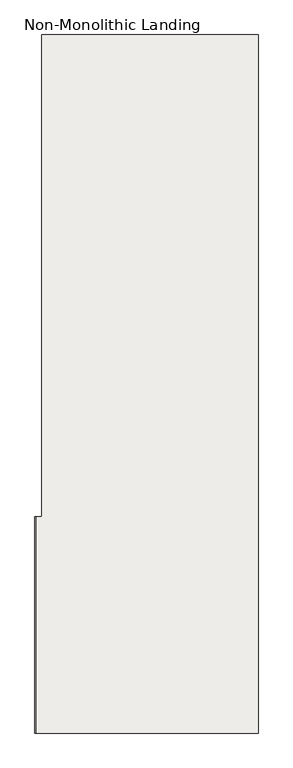
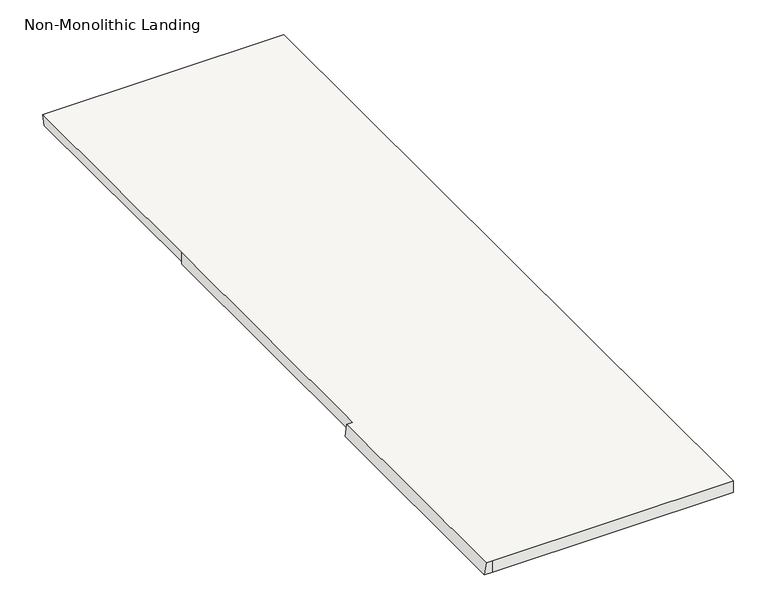
"""IFC4 building model written with IfcOpenShell, lengths in millimetres: slab geometry, Non-Monolithic Landing."""

from ifc_helpers import new_model, si_unit, origin, place, context, project, spatial, faceted_brep, source, transform, mapped, element, save


def non_monolithic_landing_cc3d4867(model_context):
    return source(origin(), model_context, "Body", "Brep", [
        faceted_brep([(-7114.5726707, -69.0804955, 1217.3913043), (-7121.7601707, -69.0804955, 1167.3913043), (-7121.7601707, -1069.1062768, 1167.3913043), (-7114.5726707, -1069.1062768, 1217.3913043), (-7089.5726707, 1160.3053702, 1217.3913043), (-7089.5726707, -69.0804955, 1217.3913043), (-7089.5726707, -1069.1062768, 1217.3913043), (-6089.5468895, -1069.1062768, 1217.3913043), (-6089.5468895, 2160.3311514, 1217.3913043), (-7089.5726707, 2160.3311514, 1217.3913043), (-7089.5726707, -69.0804955, 1167.3913043), (-7089.5726707, 1160.3053702, 1167.3913043), (-7082.3851707, 1160.3053702, 1167.3913043), (-7082.3851707, 2160.3311514, 1167.3913043), (-6089.5468895, 2160.3311514, 1167.3913043), (-6089.5468895, -1069.1062768, 1167.3913043), (-7089.5726707, -1069.1062768, 1167.3913043)], [[[0, 1, 2, 3]], [[4, 5, 0, 3, 6, 7, 8, 9]], [[10, 11, 12, 13, 14, 15, 16, 2, 1]], [[5, 4, 11, 10]], [[0, 5, 10, 1]], [[6, 3, 2, 16]], [[7, 6, 16, 15]], [[8, 7, 15, 14]], [[9, 8, 14, 13]], [[4, 12, 11]], [[12, 4, 9, 13]]]),
    ])


if __name__ == "__main__":
    model = new_model("IFC4")
    model_context = context("Model", 3, world=origin())
    ifc_project = project(units=[si_unit("LENGTHUNIT", "METRE", prefix="MILLI")], contexts=[model_context])
    site = spatial("IfcSite", under=ifc_project)
    building = spatial("IfcBuilding", under=site)
    placement = place(None, origin())
    non_monolithic_landing_shape = non_monolithic_landing_cc3d4867(model_context)
    element("IfcSlab", 1, ObjectType="Non-Monolithic Landing", at=placement, inside=building, context=model_context, shape_type="MappedRepresentation", body=[
        mapped(non_monolithic_landing_shape, transform((0.0, 0.0, 0.0), x_axis=(1.0, 0.0, 0.0), y_axis=(0.0, 1.0, 0.0), z_axis=(0.0, 0.0, 1.0))),
    ])
    save(model, "model.ifc")
